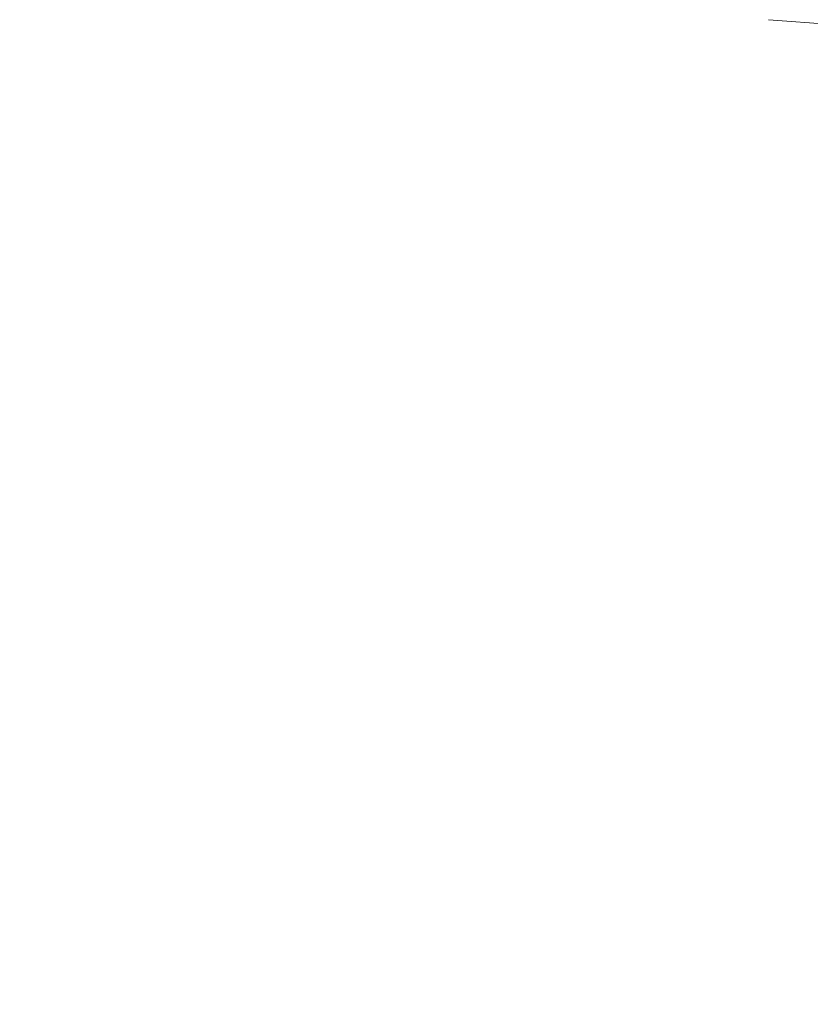
# Model space of a CAD drawing. Units: inches. Extents: x 1885 to 2748, y 783 to 2421.
# Tile 34 of 117: x 1991 to 2013, y 1531 to 1558. Entities that reach past the tile are written whole.
import ezdxf

# ---------------------------------------------------------------- set-up
doc = ezdxf.new("R2010")
doc.units = ezdxf.units.IN
doc.layers.add('A-FLOR-OPEN', color=8, linetype='Continuous', lineweight=13)
doc.layers.add('A-WALL-PATT', color=85, linetype='Continuous', lineweight=13, true_color=0x58ba48)

msp = doc.modelspace()

# ---------------------------------------------------------------- hatches: boundary and pattern name
at = {"layer": 'A-WALL-PATT'}
h = msp.add_hatch(dxfattribs=at)
h.set_pattern_fill('ANSI32', color=256)
h.paths.add_polyline_path([(2007.772, 2318.006), (1980.774, 2318.006), (1980.774, 2281.215), (1985.274, 2281.215), (1985.274, 2313.506), (2007.772, 2313.506), (2007.772, 2315.756)])
h.paths.add_polyline_path([(2094.324, 2318.006), (2067.772, 2318.006), (2067.772, 2313.506), (2094.324, 2313.506), (2094.324, 2315.756)])
h.paths.add_polyline_path([(2131.367, 2315.756), (2131.367, 2318.006), (2131.189, 2318.006), (2112.609, 2318.006), (2112.609, 2313.506), (2117.274, 2313.506), (2117.274, 2255.201), (2121.774, 2255.201), (2121.774, 2313.506), (2131.367, 2313.506)])
h.paths.add_polyline_path([(2190.512, 2318.006), (2155.367, 2318.006), (2155.367, 2313.506), (2169.774, 2313.506), (2169.774, 2229.506), (2121.774, 2229.506), (2121.774, 2233.451), (2119.524, 2233.451), (2117.274, 2233.451), (2117.274, 2201.101), (2121.774, 2201.101), (2121.774, 2225.006), (2169.774, 2225.006), (2169.774, 2165.006), (2306.274, 2165.006), (2306.274, 2066.006), (2310.774, 2066.006), (2344.274, 2066.006), (2486.274, 2066.006), (2486.274, 1886.006), (2483.02, 1886.006), (2483.02, 1881.506), (2486.274, 1881.506), (2486.274, 1880.678), (2490.774, 1880.678), (2490.774, 2070.506), (2344.274, 2070.506), (2310.774, 2070.506), (2310.774, 2165.006), (2310.774, 2173.636), (2308.524, 2173.636), (2306.274, 2173.636), (2306.274, 2169.506), (2174.274, 2169.506), (2174.274, 2313.506), (2190.512, 2313.506), (2190.512, 2315.756)])
h.paths.add_polyline_path([(1985.274, 2221.215), (1980.774, 2221.215), (1980.774, 2165.006), (1992.774, 2165.006), (1992.774, 2141.927), (1997.274, 2141.927), (1997.274, 2165.006), (2117.274, 2165.006), (2117.274, 2163.126), (2121.774, 2163.126), (2121.774, 2172.734), (2119.524, 2172.734), (2117.274, 2172.734), (2117.274, 2169.506), (1985.274, 2169.506)])
h.paths.add_polyline_path([(1997.274, 2105.927), (1992.774, 2105.927), (1992.774, 2070.506), (2016.774, 2070.506), (2016.774, 2059.123), (2019.024, 2059.123), (2021.274, 2059.123), (2021.274, 2070.506), (2117.274, 2070.506), (2117.274, 2022.506), (2114.423, 2022.506), (2114.423, 2018.006), (2123.627, 2018.006), (2123.627, 2020.256), (2123.627, 2022.506), (2121.774, 2022.506), (2121.774, 2142.587), (2119.524, 2142.587), (2117.274, 2142.587), (2117.274, 2075.006), (1997.274, 2075.006)])
h.paths.add_polyline_path([(2092.029, 2020.256), (2092.029, 2022.506), (2021.274, 2022.506), (2021.274, 2035.123), (2016.774, 2035.123), (2016.774, 2018.006), (2016.774, 1978.784), (2021.274, 1978.784), (2021.274, 2018.006), (2092.029, 2018.006)])
h.paths.add_polyline_path([(2260.938, 2022.506), (2153.105, 2022.506), (2153.105, 2020.256), (2153.105, 2018.006), (2155.274, 2018.006), (2155.274, 1886.006), (2107.629, 1886.006), (2107.629, 1881.506), (2182.911, 1881.506), (2182.911, 1883.756), (2182.911, 1886.006), (2159.774, 1886.006), (2159.774, 2018.006), (2260.938, 2018.006), (2260.938, 2020.256)])
h.paths.add_polyline_path([(2047.629, 1883.756), (2047.629, 1886.006), (2021.274, 1886.006), (2021.274, 1918.784), (2019.024, 1918.784), (2016.774, 1918.784), (2016.774, 1881.506), (2047.629, 1881.506)])
h.paths.add_polyline_path([(2306.361, 1883.756), (2306.361, 1886.006), (2296.274, 1886.006), (2296.274, 1982.006), (2316.535, 1982.006), (2316.535, 1984.256), (2316.535, 1986.506), (2296.274, 1986.506), (2296.274, 2022.506), (2289.276, 2022.506), (2289.276, 2018.006), (2291.774, 2018.006), (2291.774, 1886.006), (2242.911, 1886.006), (2242.911, 1881.506), (2306.361, 1881.506)], flags=17)
h.paths.add_polyline_path([(1985.274, 1843.006), (2021.6, 1843.006), (2021.534, 1845.441), (2021.477, 1847.506), (1980.774, 1847.506), (1980.774, 1809.446), (1985.274, 1809.446)])
h.paths.add_polyline_path([(2131.482, 1845.256), (2131.482, 1847.506), (2081.534, 1847.506), (2081.534, 1843.006), (2117.274, 1843.006), (2117.274, 1784.147), (2119.524, 1784.147), (2121.774, 1784.147), (2121.774, 1843.006), (2131.482, 1843.006)])
h.paths.add_polyline_path([(2203.886, 1847.506), (2155.482, 1847.506), (2155.482, 1843.006), (2169.774, 1843.006), (2169.774, 1759.006), (2121.774, 1759.006), (2121.774, 1761.457), (2117.274, 1761.457), (2117.274, 1730.429), (2121.774, 1730.429), (2121.774, 1754.506), (2177.421, 1754.506), (2177.421, 1756.756), (2177.421, 1759.006), (2174.274, 1759.006), (2174.274, 1843.006), (2203.886, 1843.006)])
h.paths.add_polyline_path([(2335.554, 1845.256), (2335.554, 1847.506), (2239.886, 1847.506), (2239.886, 1843.006), (2306.274, 1843.006), (2306.274, 1759.006), (2199.486, 1759.006), (2199.486, 1754.506), (2310.774, 1754.506), (2310.774, 1843.006), (2335.554, 1843.006)])
h.paths.add_polyline_path([(2348.774, 2022.506), (2344.274, 2022.506), (2344.274, 1986.506), (2341.681, 1986.506), (2341.681, 1982.006), (2344.274, 1982.006), (2344.274, 1886.006), (2330.361, 1886.006), (2330.361, 1881.506), (2361.627, 1881.506), (2361.627, 1883.756), (2361.627, 1886.006), (2348.774, 1886.006)], flags=17)
h.paths.add_polyline_path([(2283.251, 2315.756), (2283.251, 2318.006), (2238.512, 2318.006), (2238.512, 2313.506), (2283.251, 2313.506)], flags=17)
h.paths.add_polyline_path([(2363.274, 2348.006), (2388.677, 2348.006), (2388.677, 2350.256), (2388.677, 2352.506), (2358.774, 2352.506), (2358.774, 2348.006), (2358.774, 2318.006), (2344.481, 2318.006), (2344.481, 2313.506), (2358.774, 2313.506), (2358.774, 2229.506), (2310.774, 2229.506), (2310.774, 2231.952), (2306.274, 2231.952), (2306.274, 2205.611), (2310.774, 2205.611), (2310.774, 2225.006), (2358.774, 2225.006), (2358.774, 2211.506), (2452.329, 2211.506), (2452.329, 2213.756), (2452.329, 2216.006), (2363.274, 2216.006), (2363.274, 2318.006)])
h.paths.add_polyline_path([(2310.774, 2313.506), (2320.481, 2313.506), (2320.481, 2315.756), (2320.481, 2318.006), (2302.728, 2318.006), (2302.728, 2313.506), (2306.274, 2313.506), (2306.274, 2251.076), (2310.774, 2251.076)], flags=17)
h.paths.add_polyline_path([(2490.774, 2352.506), (2486.274, 2352.506), (2448.677, 2352.506), (2448.677, 2348.006), (2486.274, 2348.006), (2486.274, 2318.006), (2486.274, 2216.006), (2481.78, 2216.006), (2481.78, 2211.506), (2486.274, 2211.506), (2486.274, 2165.006), (2493.289, 2165.006), (2493.289, 2167.256), (2493.289, 2169.506), (2490.774, 2169.506), (2490.774, 2313.506), (2494.429, 2313.506), (2494.429, 2318.006), (2490.774, 2318.006)])
h.paths.add_polyline_path([(2534.653, 2318.006), (2515.691, 2318.006), (2515.691, 2313.506), (2534.653, 2313.506), (2534.653, 2315.756)])
h.paths.add_polyline_path([(2618.274, 2318.006), (2594.653, 2318.006), (2594.653, 2313.506), (2613.774, 2313.506), (2613.774, 2281.706), (2618.274, 2281.706)])
h.paths.add_polyline_path([(2618.274, 2221.706), (2613.774, 2221.706), (2613.774, 2169.506), (2554.019, 2169.506), (2554.019, 2165.006), (2613.774, 2165.006), (2613.774, 2152.878), (2618.274, 2152.878)])
h.paths.add_polyline_path([(2618.274, 2128.878), (2616.024, 2128.878), (2613.774, 2128.878), (2613.774, 2117.006), (2529.774, 2117.006), (2529.774, 2165.006), (2532.848, 2165.006), (2532.848, 2169.506), (2522.867, 2169.506), (2522.867, 2165.006), (2525.274, 2165.006), (2525.274, 2117.006), (2525.274, 2112.506), (2525.274, 2108.576), (2529.774, 2108.576), (2529.774, 2112.506), (2613.774, 2112.506), (2613.774, 2080.19), (2618.274, 2080.19)])
h.paths.add_polyline_path([(2618.274, 2044.19), (2616.024, 2044.19), (2613.774, 2044.19), (2613.774, 2015.506), (2529.774, 2015.506), (2529.774, 2088.582), (2527.524, 2088.582), (2525.274, 2088.582), (2525.274, 2011.006), (2613.774, 2011.006), (2613.774, 1956.755), (2618.274, 1956.755)])
h.paths.add_polyline_path([(2618.274, 1881.506), (2618.274, 1896.755), (2613.774, 1896.755), (2613.774, 1881.506), (2613.774, 1847.506), (2592.715, 1847.506), (2592.715, 1843.006), (2613.774, 1843.006), (2613.774, 1765.006), (2613.774, 1760.506), (2609.621, 1760.506), (2609.621, 1756.006), (2613.774, 1756.006), (2613.774, 1660.006), (2608.544, 1660.006), (2608.544, 1655.506), (2613.774, 1655.506), (2613.774, 1508.158), (2618.274, 1508.158)])
h.paths.add_polyline_path([(2565.774, 1843.006), (2568.997, 1843.006), (2568.997, 1847.506), (2490.774, 1847.506), (2490.774, 1849.7), (2488.524, 1849.7), (2486.274, 1849.7), (2486.274, 1847.506), (2477.274, 1847.506), (2477.274, 1838.506), (2477.274, 1821.493), (2486.274, 1821.493), (2486.274, 1838.506), (2561.274, 1838.506), (2561.274, 1765.006), (2486.274, 1765.006), (2486.274, 1786.157), (2477.274, 1786.157), (2477.274, 1765.006), (2477.274, 1756.006), (2486.274, 1756.006), (2565.774, 1756.006), (2585.621, 1756.006), (2585.621, 1758.256), (2585.621, 1760.506), (2565.774, 1760.506), (2565.774, 1765.006)])
h.paths.add_polyline_path([(2486.274, 1651.006), (2561.274, 1651.006), (2561.274, 1567.006), (2486.274, 1567.006), (2486.274, 1591.321), (2477.274, 1591.321), (2477.274, 1567.006), (2477.274, 1558.006), (2477.274, 1555.439), (2481.774, 1555.439), (2481.774, 1558.006), (2568.653, 1558.006), (2568.653, 1560.256), (2568.653, 1562.506), (2565.774, 1562.506), (2565.774, 1655.506), (2584.544, 1655.506), (2584.544, 1657.756), (2584.544, 1660.006), (2565.774, 1660.006), (2486.274, 1660.006), (2477.274, 1660.006), (2477.274, 1651.006), (2477.274, 1632.989), (2486.274, 1632.989)])
h.paths.add_polyline_path([(2449.967, 1883.756), (2449.967, 1886.006), (2421.627, 1886.006), (2421.627, 1881.506), (2449.967, 1881.506)], flags=17)
h.paths.add_polyline_path([(2447.274, 1847.506), (2395.554, 1847.506), (2395.554, 1843.006), (2442.774, 1843.006), (2442.774, 1809.27), (2447.274, 1809.27)])
h.paths.add_polyline_path([(1985.274, 1749.446), (1980.774, 1749.446), (1980.774, 1694.504), (1985.274, 1694.504), (1985.274, 1694.506), (1986.897, 1694.506), (1986.897, 1697.78), (1986.897, 1699.006), (1985.274, 1699.006)])
h.paths.add_polyline_path([(2152.774, 1699.006), (2121.774, 1699.006), (2121.774, 1703.668), (2119.524, 1703.668), (2117.274, 1703.668), (2117.274, 1699.006), (2009.219, 1699.006), (2009.219, 1694.506), (2148.274, 1694.506), (2148.274, 1692.631), (2152.774, 1692.631)])
h.paths.add_polyline_path([(2016.274, 1694.506), (2011.774, 1694.506), (2011.774, 1558.006), (2040.806, 1558.006), (2040.806, 1560.256), (2040.806, 1562.506), (2016.274, 1562.506)])
h.paths.add_polyline_path([(2152.774, 1663.017), (2150.524, 1663.017), (2148.274, 1663.017), (2148.274, 1562.506), (2100.806, 1562.506), (2100.806, 1558.006), (2165.119, 1558.006), (2165.119, 1560.256), (2165.119, 1562.506), (2152.774, 1562.506), (2152.774, 1610.506), (2224.774, 1610.506), (2224.774, 1607.99), (2229.274, 1607.99), (2229.274, 1615.006), (2152.774, 1615.006)])
h.paths.add_polyline_path([(2238.613, 1560.256), (2238.613, 1562.506), (2229.274, 1562.506), (2229.274, 1588.756), (2227.024, 1588.763), (2224.774, 1588.771), (2224.774, 1562.506), (2189.119, 1562.506), (2189.119, 1558.006), (2238.613, 1558.006)])
h.paths.add_polyline_path([(2336.024, 1560.256), (2336.024, 1562.506), (2310.774, 1562.506), (2310.774, 1656.347), (2308.524, 1656.347), (2306.274, 1656.347), (2306.274, 1562.506), (2286.613, 1562.506), (2286.613, 1558.006), (2336.024, 1558.006)])
h.paths.add_polyline_path([(2447.274, 1690.968), (2445.024, 1690.968), (2442.774, 1690.968), (2442.774, 1687.006), (2306.274, 1687.006), (2306.274, 1680.75), (2310.774, 1680.75), (2310.774, 1682.506), (2442.774, 1682.506), (2442.774, 1562.506), (2396.024, 1562.506), (2396.024, 1558.006), (2447.274, 1558.006)])
h.paths.add_polyline_path([(2447.274, 1749.27), (2445.024, 1749.27), (2442.774, 1749.27), (2442.774, 1717.232), (2447.274, 1717.232)])
h.paths.add_polyline_path([(2044.674, 1521.756), (2044.674, 1524.006), (2007.274, 1524.006), (2007.274, 1503.49), (2009.524, 1503.49), (2011.774, 1503.49), (2011.774, 1519.506), (2044.674, 1519.506)])
h.paths.add_polyline_path([(2177.969, 1521.756), (2177.969, 1524.006), (2104.674, 1524.006), (2104.674, 1519.506), (2145.774, 1519.506), (2145.774, 1387.506), (2143.37, 1387.506), (2143.37, 1383.006), (2251.585, 1383.006), (2251.585, 1385.256), (2251.585, 1387.506), (2150.274, 1387.506), (2150.274, 1519.506), (2177.969, 1519.506)])
h.paths.add_polyline_path([(2298.704, 1524.006), (2237.969, 1524.006), (2237.969, 1519.506), (2282.274, 1519.506), (2282.274, 1387.506), (2279.683, 1387.506), (2279.683, 1383.006), (2286.774, 1383.006), (2286.774, 1419.006), (2312.451, 1419.006), (2312.451, 1421.256), (2312.451, 1423.506), (2286.774, 1423.506), (2286.774, 1519.506), (2298.704, 1519.506), (2298.704, 1521.722)], flags=17)
h.paths.add_polyline_path([(2361.897, 1521.756), (2361.897, 1524.006), (2322.704, 1524.006), (2322.704, 1519.506), (2334.774, 1519.506), (2334.774, 1423.506), (2331.93, 1423.506), (2331.93, 1419.006), (2334.774, 1419.006), (2334.774, 1387.506), (2334.774, 1383.228), (2339.274, 1383.228), (2339.274, 1387.506), (2339.274, 1519.506), (2361.897, 1519.506)], flags=17)
h.paths.add_polyline_path([(2447.274, 1521.756), (2447.274, 1524.006), (2421.897, 1524.006), (2421.897, 1519.506), (2447.274, 1519.506)], flags=17)
h.paths.add_polyline_path([(2481.774, 1529.6), (2479.524, 1529.6), (2477.274, 1529.6), (2477.274, 1524.006), (2474.489, 1524.006), (2474.489, 1519.506), (2477.274, 1519.506), (2477.274, 1334.506), (2296.774, 1334.506), (2296.774, 1240.506), (2160.274, 1240.506), (2160.274, 1180.506), (2112.274, 1180.506), (2112.274, 1207.692), (2110.024, 1207.692), (2107.774, 1207.692), (2107.774, 1171.609), (2112.274, 1171.609), (2112.274, 1176.006), (2160.274, 1176.006), (2160.274, 1092.006), (2144.221, 1092.006), (2144.221, 1087.506), (2189.497, 1087.506), (2189.497, 1089.756), (2189.497, 1092.006), (2164.774, 1092.006), (2164.774, 1236.006), (2296.774, 1236.006), (2296.774, 1231.912), (2301.274, 1231.912), (2301.274, 1330.006), (2481.774, 1330.006), (2481.774, 1387.506)])
h.paths.add_polyline_path([(2618.274, 1448.158), (2613.774, 1448.158), (2613.774, 1382.506), (2529.774, 1382.506), (2525.274, 1382.506), (2525.274, 1307.062), (2529.774, 1307.062), (2529.774, 1378.006), (2613.774, 1378.006), (2613.774, 1354.988), (2618.274, 1354.988)])
h.paths.add_polyline_path([(2618.274, 1318.988), (2613.774, 1318.988), (2613.774, 1281.006), (2529.774, 1281.006), (2529.774, 1283.786), (2527.524, 1283.786), (2525.274, 1283.786), (2525.274, 1228.506), (2516.794, 1228.506), (2516.794, 1224.006), (2533.484, 1224.006), (2533.484, 1226.256), (2533.484, 1228.506), (2529.774, 1228.506), (2529.774, 1276.506), (2613.774, 1276.506), (2613.774, 1266.02), (2618.274, 1266.02)])
h.paths.add_polyline_path([(2618.274, 1134.964), (2613.774, 1134.964), (2613.774, 1092.006), (2594.545, 1092.006), (2594.545, 1087.506), (2618.274, 1087.506)])
h.paths.add_polyline_path([(2534.545, 1092.006), (2509.765, 1092.006), (2509.765, 1087.506), (2534.545, 1087.506), (2534.545, 1089.756)])
h.paths.add_polyline_path([(2481.274, 1224.006), (2484.117, 1224.006), (2484.117, 1226.256), (2484.117, 1228.506), (2476.774, 1228.506), (2476.774, 1198.506), (2471.61, 1198.506), (2471.61, 1194.006), (2476.774, 1194.006), (2476.774, 1062.006), (2436.894, 1062.006), (2436.894, 1057.506), (2476.774, 1057.506), (2481.274, 1057.506), (2481.274, 1062.006), (2481.274, 1087.506), (2485.354, 1087.506), (2485.354, 1089.756), (2485.354, 1092.006), (2481.274, 1092.006), (2481.274, 1117.506)])
h.paths.add_polyline_path([(2439.898, 1198.506), (2349.274, 1198.506), (2349.274, 1194.006), (2349.274, 1180.506), (2301.274, 1180.506), (2301.274, 1201.896), (2299.024, 1201.896), (2296.774, 1201.896), (2296.774, 1172.335), (2299.024, 1172.335), (2301.274, 1172.335), (2301.274, 1176.006), (2349.274, 1176.006), (2349.274, 1092.006), (2334.452, 1092.006), (2334.452, 1087.506), (2349.274, 1087.506), (2349.274, 1057.506), (2353.774, 1057.506), (2376.894, 1057.506), (2376.894, 1059.756), (2376.894, 1062.006), (2353.774, 1062.006), (2353.774, 1087.506), (2353.774, 1180.506), (2353.774, 1194.006), (2439.898, 1194.006), (2439.898, 1196.256)])
h.paths.add_polyline_path([(2270.596, 1089.756), (2270.596, 1092.006), (2249.497, 1092.006), (2249.497, 1087.506), (2270.596, 1087.506)], flags=17)
h.paths.add_polyline_path([(2310.452, 1092.006), (2301.274, 1092.006), (2301.274, 1153.292), (2296.774, 1153.292), (2296.774, 1092.006), (2293.786, 1092.006), (2293.786, 1087.506), (2310.452, 1087.506), (2310.452, 1089.756)], flags=17)
h.paths.add_polyline_path([(2112.274, 1150.328), (2110.024, 1150.328), (2107.774, 1150.328), (2107.774, 1092.006), (2104.465, 1092.006), (2104.465, 1087.506), (2120.221, 1087.506), (2120.221, 1089.756), (2120.221, 1092.006), (2112.274, 1092.006)])
h.paths.add_polyline_path([(2082.172, 1092.006), (2058.144, 1092.006), (2058.144, 1087.506), (2082.172, 1087.506), (2082.172, 1089.756)])
h.paths.add_polyline_path([(1975.774, 1145.638), (1971.274, 1145.638), (1971.274, 1087.506), (1980.774, 1087.506), (1998.144, 1087.506), (1998.144, 1089.756), (1998.144, 1092.006), (1985.274, 1092.006), (1975.774, 1092.006)])
h.paths.add_polyline_path([(2112.274, 1244.385), (2110.024, 1244.385), (2107.774, 1244.385), (2107.774, 1240.506), (1992.274, 1240.506), (1992.274, 1271.008), (1987.774, 1271.008), (1987.774, 1240.506), (1980.774, 1240.506), (1975.774, 1240.506), (1971.274, 1240.506), (1971.274, 1205.638), (1975.774, 1205.638), (1975.774, 1236.006), (2107.774, 1236.006), (2107.774, 1233.444), (2112.274, 1233.444), (2112.274, 1236.006)])
h.paths.add_polyline_path([(2112.274, 1383.006), (2114.783, 1383.006), (2114.783, 1385.256), (2114.783, 1387.506), (2102.476, 1387.506), (2102.476, 1383.006), (2107.774, 1383.006), (2107.774, 1335.006), (2011.774, 1335.006), (2011.774, 1349.939), (2007.274, 1349.939), (2007.274, 1335.006), (1987.774, 1335.006), (1987.774, 1330.506), (1987.774, 1307.008), (1992.274, 1307.008), (1992.274, 1330.506), (2007.274, 1330.506), (2107.774, 1330.506), (2107.774, 1264.711), (2112.274, 1264.711)])
h.paths.add_polyline_path([(2077.857, 1387.506), (2011.774, 1387.506), (2011.774, 1390.036), (2009.524, 1390.036), (2007.274, 1390.036), (2007.274, 1373.939), (2011.774, 1373.939), (2011.774, 1383.006), (2077.857, 1383.006)])
h.paths.add_polyline_path([(2011.774, 1443.49), (2007.274, 1443.49), (2007.274, 1410.248), (2011.774, 1410.248)])

# ---------------------------------------------------------------- linework, layer by layer
at = {"layer": 'A-FLOR-OPEN'}
msp.add_line((2447.274, 1524.006), (2011.774, 1558.006), dxfattribs=at)

doc.saveas('drawing.dxf')
